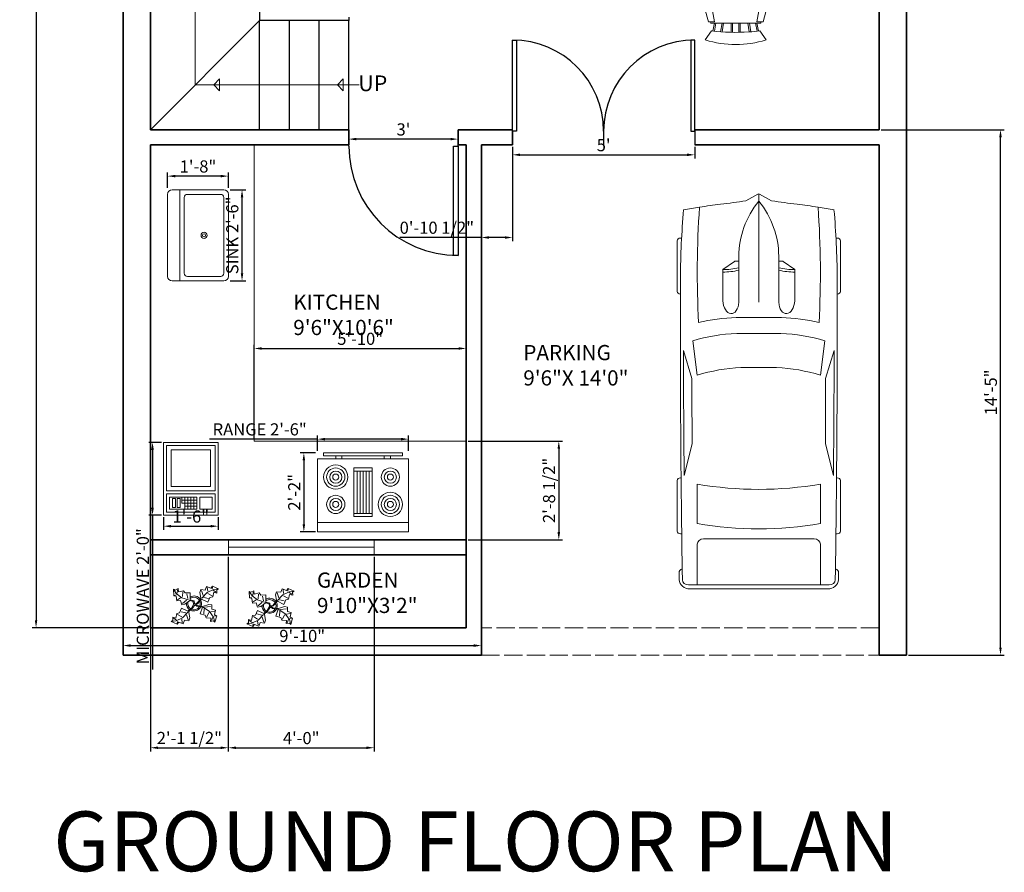
# Model space of a CAD drawing. Units: inches. Extents: x 2170 to 3011, y 1733 to 2338.
# Tile 1 of 5: x 2172 to 2496, y 1733 to 2014. Entities that reach past the tile are written whole.
import ezdxf

# ---------------------------------------------------------------- set-up
doc = ezdxf.new("R2010")
doc.units = ezdxf.units.IN
doc.linetypes.add('ACAD_ISO02W100', pattern=[15, 12, -3])
for name, color, linetype, lineweight in [('A-ANNO-SYMB', 2, 'Continuous', 13), ('A-AREA-IDEN', 4, 'Continuous', 18), ('A-EQPM', 20, 'Continuous', 18), ('A-FLOR-CASE', 20, 'Continuous', 20), ('A-FLOR-FIXT', 20, 'Continuous', 18), ('A-WALL', 7, 'Continuous', 35), ('A-WALL-OVHD', 7, 'ACAD_ISO02W100', 18), ('car', 81, 'Continuous', 13), ('dim', 11, 'Continuous', 18), ('door', 6, 'Continuous', 25), ('furnitures', 20, 'Continuous', 18), ('L-PLNT', 81, 'Continuous', 13), ('stairs', 150, 'Continuous', 25), ('text', 4, 'Continuous', 18), ('window', 3, 'Continuous', 20)]:
    doc.layers.add(name, color=color, linetype=linetype, lineweight=lineweight)
doc.styles.get("Standard").update_dxf_attribs({"font": 'arial.ttf'})
doc.dimstyles.new('ISO-25', dxfattribs={"dimtxt": 4, "dimasz": 2.5, "dimexe": 1.25, "dimexo": 0.625, "dimtad": 1, "dimlunit": 3, "dimtxsty": 'Standard', "dimcen": 2.5, "dimadec": 0, "dimazin": 0, "dimtfac": 1, "dimtmove": 0, "dimatfit": 3, "dimfxl": 1, "dimarcsym": 0})

# ---------------------------------------------------------------- blocks, each defined once
blk = doc.blocks.new('*U4')
for p, q in [((0, 0), (0, -6)), ((40, 0), (40, -6))]:
    blk.add_line(p, q)
blk.add_lwpolyline([(0, 0), (0, 40), (1.75, 40), (1.75, 0)], close=True)
blk.add_arc((0, 0), 40, 0, 90)
blk = doc.blocks.new('*U2')
for p, q in [((0, 0), (0, -6)), ((40, 0), (40, -6))]:
    blk.add_line(p, q)
blk.add_lwpolyline([(0, 0), (0, 40), (1.75, 40), (1.75, 0)], close=True)
blk.add_arc((0, 0), 40, 0, 90)
blk = doc.blocks.new('*U3')
for p, q in [((0, 0), (0, -6)), ((-40, 0), (-40, -6))]:
    blk.add_line(p, q)
blk.add_lwpolyline([(0, 0), (0, 40), (-1.75, 40), (-1.75, 0)], close=True)
blk.add_arc((0, 0), 40, 90, 180)
blk = doc.blocks.new('Range-Oven - 30 in top')
for p, q in [((0, -3), (30, -3)), ((12, -6), (18, -6)), ((13, -20), (13, -6)), ((14, -6), (14, -20)), ((15, -20), (15, -6)), ((16, -6), (16, -20)), ((17, -20), (17, -6)), ((18, -20), (12, -20)), ((6, -24), (6, -25)), ((8, -25), (8, -24)), ((22, -25), (22, -24)), ((24, -24), (24, -25))]:
    blk.add_line(p, q)
for points in [[(0, -24), (0, 0), (30, 0), (30, -24)], [(12, -21), (12, -5), (18, -5), (18, -21)], [(2, -26), (2, -25), (28, -25), (28, -26)]]:
    blk.add_lwpolyline(points, close=True)
for centre, radius in [((6, -9), 4), ((6, -9), 3), ((24, -9), 3), ((6, -9), 2), ((6, -9), 1), ((24, -9), 2), ((24, -9), 1), ((6, -18), 3), ((6, -18), 2), ((24, -18), 4), ((24, -18), 3), ((24, -18), 2), ((6, -18), 1), ((24, -18), 1)]:
    blk.add_circle(centre, radius)
blk = doc.blocks.new('Microwave')
for p, q in [((18, 10), (22, 10)), ((19, 7), (19, 11)), ((20, 11), (20, 7)), ((21, 7), (21, 11)), ((22, 9), (18, 9)), ((18, 8), (22, 8)), ((22, 7), (18, 7)), ((19, 6), (19, 7)), ((20, 7), (20, 6)), ((20, 6), (18, 6))]:
    blk.add_line(p, q)
for points in [[(0, 0), (0, 18), (24, 18), (24, 0)], [(1, 1), (1, 17), (16, 17), (16, 1)], [(17, 1), (17, 17), (23, 17), (23, 1)], [(2.5, 2.5), (2.5, 15.5), (14.5, 15.5), (14.5, 2.5)], [(18, 12), (18, 16), (22, 16), (22, 12)], [(18, 2), (18, 11), (22, 11), (22, 2)], [(18.5, 4.5), (18.5, 5.5), (21.5, 5.5), (21.5, 4.5)], [(18.5, 3), (18.5, 4), (21.5, 4), (21.5, 3)]]:
    blk.add_lwpolyline(points, close=True)
blk = doc.blocks.new('Sink-single - 30 in top')
blk.add_line((-15, -3.999996), (15, -3.999996))
for points in [[(-13.5, 0), (13.5, 0)], [(-15, -18.499996), (-15, -1.5)], [(15, -1.5), (15, -18.499996)], [(-12.5, -5.499996), (12.5, -5.499996)], [(-13.5, -17.499996), (-13.5, -6.499996)], [(13.5, -6.499996), (13.5, -17.499996)], [(12.5, -18.499996), (-12.5, -18.499996)], [(13.5, -19.999996), (-13.5, -19.999996)]]:
    blk.add_lwpolyline(points)
for radius in [1, 0.5]:
    blk.add_circle((0, -11.999996), radius)
for centre, radius, start, end in [((-13.5, -1.5), 1.5, 90, 180), ((13.5, -1.5), 1.5, 0, 90), ((-12.5, -6.499996), 1, 90, 180), ((12.5, -6.499996), 1, 0, 90), ((-13.5, -18.499996), 1.5, 180, 270), ((-12.5, -17.499996), 1, 180, 270), ((12.5, -17.499996), 1, 270, 0), ((13.5, -18.499996), 1.5, 270, 0)]:
    blk.add_arc(centre, radius, start, end)
blk = doc.blocks.new('Plant - Rubber or Philodendron')
for p, q in [((-16.2005, 11.4774), (-13.9899, 8.1064)), ((-16.2005, 11.4774), (-14.8639, 10.7964)), ((-16.0159, 6.3329), (-16.2005, 11.4774)), ((-14.8639, 10.7964), (-12.6195, 11.8975)), ((-13.9899, 8.1064), (-9.5434, 4.7185)), ((-13.3174, 8.325), (-13.0735, 11.0065)), ((-12.6195, 11.8975), (-12.1909, 9.4345)), ((-12.1909, 9.4345), (-8.3829, 10.3)), ((-8.8369, 9.409), (-9.0894, 5.6095)), ((-8.3829, 10.3), (-7.0549, 8.501)), ((-7.0549, 8.501), (-3.0284, 8.6941)), ((-4.8529, 4.012), (-5.7184, 7.82)), ((-3.0284, 8.6941), (-3.0709, 3.1041)), ((4.6914, 8.8812), (5.3859, 11.2828)), ((4.6914, 8.8812), (5.5014, 4.4831)), ((5.3859, 11.2828), (8.8871, 10.7908)), ((5.9878, 10.4842), (7.1971, 6.3869)), ((10.3916, 8.7942), (6.2847, 4.4028)), ((8.8871, 10.7908), (9.9809, 13.4933)), ((9.9809, 13.4933), (13.3837, 12.301)), ((15.3859, 11.3055), (10.3916, 8.7942)), ((10.5828, 12.6946), (10.8893, 9.7953)), ((14.2977, 6.1031), (10.9934, 7.9956)), ((13.3837, 12.301), (14.68, 13.9039)), ((14.5816, 13.2037), (14.3848, 11.8033)), ((14.68, 13.9039), (19.3848, 11.8146)), ((15.7909, 9.1065), (14.8995, 5.3044)), ((15.2875, 10.6053), (17.5907, 9.2105)), ((19.3848, 11.8146), (15.3859, 11.3055)), ((18.1925, 8.4119), (15.7909, 9.1065)), ((19.3848, 11.8146), (18.1868, 10.9119)), ((18.1868, 10.9119), (18.1925, 8.4119)), ((-14.0069, 5.8704), (-16.0159, 6.3329)), ((-15.3434, 6.5514), (-13.9984, 6.9884)), ((-13.5868, 2.2894), (-14.0069, 5.8704)), ((-10.6784, 2.491), (-13.5868, 2.2894)), ((-13.1329, 3.1804), (-10.6614, 4.727)), ((-9.5858, -0.8715), (-10.6784, 2.491)), ((-9.5434, 4.7185), (-4.1917, 2.9888)), ((-9.1318, 0.0195), (-5.9793, 2.9025)), ((-7.1228, -0.443), (-3.5248, 2.2131)), ((-3.5248, 2.2131), (-3.3011, 2.4355)), ((-3.3011, 2.4355), (-0.5306, 1.7947)), ((-3.0709, 3.1041), (0.0797, 2.3163)), ((-0.5306, 1.7947), (-0.2255, -0.5527)), ((-0.5306, 1.7947), (-0.5306, 1.7947)), ((0.0797, 2.3163), (0.4866, -0.031)), ((0.4866, -0.031), (2.1141, 0.2298)), ((2.1141, 0.2298), (5.4346, 3.9146)), ((6.1032, 3.6844), (2.8262, -0.031)), ((5.4346, 3.9146), (5.5014, 4.4831)), ((11.1089, 1.1958), (6.1032, 3.6844)), ((7.7005, 4.8881), (11.5025, 3.9967)), ((12.7005, 4.8994), (11.1089, 1.1958)), ((14.8995, 5.3044), (12.7005, 4.8994)), ((-14.4141, -11.4699), (-13.5228, -7.6679)), ((-13.5228, -7.6679), (-11.3237, -7.2629)), ((-11.3237, -7.2629), (-9.7321, -3.5593)), ((-6.3237, -7.2516), (-10.1257, -6.3602)), ((-9.7321, -3.5593), (-4.7264, -6.0479)), ((-7.1228, -0.443), (-9.5858, -0.8715)), ((-9.0148, -11.1577), (-4.9047, -6.8122)), ((-2.019, -3.6148), (-4.7264, -6.0479)), ((-4.1246, -6.8466), (-4.0579, -6.2781)), ((-3.3146, -11.2447), (-4.1246, -6.8466)), ((-4.0579, -6.2781), (-0.9375, -3.1608)), ((-2.019, -3.6148), (-0.2255, -0.5527)), ((-0.9375, -3.1608), (0.5883, -0.8135)), ((0.5883, -0.8135), (2.2447, -2.0916)), ((2.8262, -0.031), (1.3003, -0.5527)), ((1.3003, -0.5527), (2.4193, -1.4655)), ((2.2447, -2.0916), (6.7108, -2.6626)), ((2.4193, -1.4655), (6.895, -2.1175)), ((4.943, -7.9659), (6.7108, -2.6626)), ((11.6605, -0.5413), (6.895, -2.1175)), ((12.3677, -6.1981), (7.219, -2.6772)), ((8.125, -4.0768), (7.7715, -7.9659)), ((8.3544, -2.7453), (13.1973, -2.1704)), ((10.2463, -10.4408), (11.6605, -6.9053)), ((11.6605, -0.5413), (14.1354, -0.8948)), ((15.5496, -10.7943), (12.3677, -6.1981)), ((16.2567, -5.8446), (13.4283, -6.5517)), ((14.1354, -0.8948), (14.1354, -4.4304)), ((14.1354, -4.4304), (16.9638, -5.1375)), ((16.9638, -5.1375), (16.2567, -8.673)), ((-18.008, -14.1781), (-16.8101, -13.2754)), ((-18.008, -14.1781), (-14.0091, -13.669)), ((-13.3032, -16.2674), (-18.008, -14.1781)), ((-16.8157, -10.7754), (-14.4141, -11.4699)), ((-16.8101, -13.2754), (-16.8157, -10.7754)), ((-13.9107, -12.9688), (-16.2139, -11.574)), ((-14.0091, -13.669), (-9.0148, -11.1577)), ((-12.0069, -14.6645), (-13.3032, -16.2674)), ((-13.2048, -15.5672), (-13.008, -14.1668)), ((-12.921, -8.4665), (-9.6166, -10.359)), ((-8.6042, -15.8568), (-12.0069, -14.6645)), ((-9.206, -15.0581), (-9.5126, -12.1588)), ((-7.5103, -13.1543), (-8.6042, -15.8568)), ((-4.0092, -13.6463), (-7.5103, -13.1543)), ((-4.611, -12.8477), (-5.8203, -8.7504)), ((-3.3146, -11.2447), (-4.0092, -13.6463)), ((8.8321, -9.0266), (4.943, -7.9659)), ((9.5392, -11.1479), (8.8321, -9.0266)), ((13.4283, -11.5015), (9.5392, -11.1479)), ((13.0748, -13.9763), (13.4283, -11.5015)), ((15.5496, -13.6228), (13.0748, -13.9763)), ((14.8425, -10.7943), (13.7819, -13.2692)), ((16.6103, -14.6834), (15.5496, -10.7943)), ((16.6103, -14.6834), (15.5496, -13.6228)), ((17.3174, -9.7337), (15.9032, -9.7337)), ((16.2567, -8.673), (18.0245, -9.7337)), ((18.0245, -9.7337), (16.6103, -14.6834))]:
    blk.add_line(p, q)
for centre, radius, start, end in [((0.0308, 0.1664), 6, 178.6147, 235.1169), ((0.0308, 0.1664), 5, 168.1647, 238.6725), ((0, 0), 6.1275, 34.37569, 120.1028), ((-0.0601, -0.2075), 5.2461, 33.82192, 124.9414), ((-0.2664, 0.1682), 5.2775, 338.4094, 20.03007), ((-0.098, 0.1364), 6.1288, 341.2017, 26.09184), ((-0.0234, 0.3825), 6.1492, 242.5812, 331.2714), ((-0.1102, 0.4886), 5.2883, 247.3711, 327.472)]:
    blk.add_arc(centre, radius, start, end)
blk = doc.blocks.new('Chair - Rocking')
for p, q in [((-8, -4.5), (-10, -1.5)), ((8, -4.5), (10, -1.5)), ((-7.5, -4.5), (-7, -7)), ((-6.5, -7), (-7.02225, -4.43)), ((-4.5, -7), (-4.96674, -4.19951)), ((-4, -7), (-4.40532, -4.16272)), ((-1.5, -4.05012), (-1.5, -7)), ((-1, -7), (-1, -4.05012)), ((1, -7), (1, -4.04655)), ((1.5, -4.05012), (1.5, -7)), ((4, -7), (4.40187, -4.18694)), ((4.5, -7), (4.96761, -4.19437)), ((6.5, -7), (7, -4.4057)), ((7.5, -4.5), (7, -7)), ((-9, -7.5), (-12, -18.49999)), ((-7, -7.5), (-9, -7.5)), ((-9, -18.49999), (-7, -7.5)), ((-8.23428, -6.99939), (-8.3093, -7.47958)), ((-8.23041, -7), (8.23915, -7)), ((7, -7.5), (9, -7.5)), ((9, -18.49999), (7, -7.5)), ((8.31071, -7.48854), (8.23449, -7.00073)), ((9, -7.5), (12, -18.49999)), ((-10.36644, -20.64523), (-10.5, -21.49999)), ((-9, -22.49999), (-9.5, -26.49999)), ((0, -22.49999), (-9.5, -22.49999)), ((-8, -26.49999), (-7.5, -22.49999)), ((0, -22.49999), (9.5, -22.49999)), ((8, -26.49999), (7.5, -22.49999)), ((9, -22.49999), (9.5, -26.49999)), ((10.5, -21.49999), (10.3575, -20.58798)), ((-9.5, -26.49999), (-8, -26.49999)), ((9.5, -26.49999), (8, -26.49999))]:
    blk.add_line(p, q)
for centre, radius, start, end in [((0, -34.08333), 34.08333, 72.93847, 107.0615), ((0, -68.25004), 64.25, 93.92211, 97.15267), ((0, -68.25004), 64.25, 82.84733, 93.92211), ((-10.5, -18.99999), 1.58114, 161.5651, 18.43495), ((10.5, -18.99999), 1.58114, 161.5651, 18.43495), ((-9.5, -21.49999), 1, 180, 270), ((9.5, -21.49999), 1, 270, 0)]:
    blk.add_arc(centre, radius, start, end)
blk = doc.blocks.new('*U21')
for p, q in [((46.55, 38.89), (22.35, 38.89)), ((136.7, 38.89), (160.9, 38.89)), ((21.1, 37.41), (21.1, 36.83)), ((47.8, 37.39), (47.8, 37.41)), ((87.99, 31.87), (74.76, 35.92)), ((134.31, 35.6), (119.29, 31.78)), ((135.45, 37.07), (135.45, 37.41)), ((162.15, 37.41), (162.15, 36.77)), ((186.47, -33.5), (186.47, 33.5)), ((70.03, 31.54), (86.41, 29.35)), ((138.42, 29.35), (157.25, 29.35)), ((186.47, 29.35), (167.01, 29.35)), ((188.4, -32.76), (188.4, 32.76)), ((164.52, 26.39), (164.52, -26.39)), ((32.27, 11.63), (36.13, 17.17)), ((36.13, 17.17), (50.94, 17.17)), ((29.77, 9.51), (51.68, 9.51)), ((32.12, 9.51), (32.12, 11.15)), ((58.92, -10.77), (58.92, 10.77)), ((66.55, -10.53), (66.55, 10.53)), ((186.47, -10.53), (186.47, 10.53)), ((3.27, 6.13), (0.1, 0.41)), ((82.74, 8.5), (82.74, -8.5)), ((0, 0), (51.68, 0)), ((0.1, -0.41), (3.27, -6.13)), ((29.77, -9.51), (51.68, -9.51)), ((32.12, -9.51), (32.12, -11.15)), ((32.27, -11.63), (36.13, -17.17)), ((36.13, -17.17), (50.94, -17.17)), ((86.41, -29.35), (70.03, -31.54)), ((87.99, -31.87), (74.76, -35.92)), ((134.31, -35.6), (119.29, -31.78)), ((157.25, -29.35), (138.42, -29.35)), ((167.01, -29.35), (186.47, -29.35)), ((21.1, -37.41), (21.1, -36.83)), ((47.8, -37.39), (47.8, -37.41)), ((135.45, -37.07), (135.45, -37.41)), ((162.15, -37.41), (162.15, -36.77)), ((46.55, -38.89), (22.35, -38.89)), ((136.7, -38.89), (160.9, -38.89))]:
    blk.add_line(p, q)
for centre, major_axis, ratio, start_param, end_param in [((22.35, 37.41), (0, -1.48), 0.842304, 3.141593, 4.712389), ((46.55, 37.41), (0, 1.48), 0.842304, -1.570796, 0), ((136.7, 37.41), (0, -1.48), 0.842304, 3.141593, 4.712389), ((160.9, 37.41), (0, 1.48), 0.842304, -1.570796, 0), ((180.63, 35.84), (0, 2.22), 0.842304, -0.013017, 1.249894), ((64.48, -10556.36), (0, 10595.31), 0.842304, -0.013397, -0.013017), ((183.98, 32.76), (0, -5.25), 0.842304, 1.570796, 3.128196), ((266.03, -27.52), (0, 313.31), 0.842304, 1.367076, 1.39176), ((41.19, -490.86), (0, 528.23), 0.842304, 0.00281, 0.075598), ((64.48, -10555.62), (0, 10593.03), 0.842304, -0.013397, 0.002797), ((64.48, -10555.62), (0, -10591.55), 0.842304, 3.133765, 3.140441), ((183.98, 33.5), (0, -2.96), 0.842304, 1.570796, 3.128196), ((259.18, -27.52), (0, -305.3), 0.842304, 4.528606, 4.561838), ((37.47, -593.96), (0, -623.33), 0.842304, 3.096046, 3.200911), ((134.4, 5.39), (0, -89.78), 0.842304, 4.449482, 4.652344), ((135.29, 5.39), (0, 81.77), 0.842304, 1.245306, 1.50788), ((149.6, 2.8), (0, -79.58), 0.842304, 4.372215, 4.640744), ((95.79, -3666.35), (0, -3698.24), 0.842304, 3.134049, 3.144098), ((17.08, 0), (0, 147.02), 0.842304, 4.511394, 4.913384), ((35.91, 0), (0, 147.02), 0.842304, 4.511394, 4.913384), ((167.01, 26.39), (0, 2.96), 0.842304, 0, 1.570796), ((-204.49, 52.4), (0, -250.96), 0.842304, 1.385369, 1.434372), ((13.04, 17.01), (0, 27.42), 0.842304, 4.435146, 4.718221), ((14.2, 17.01), (0, 27.42), 0.842304, 4.435146, 4.718221), ((50.79, 13.34), (6.34, -0.36), 0.603834, -1.395552, 1.581315), ((29.77, -46.66), (0, 56.17), 0.842304, 0, 0.590319), ((32.75, 11.15), (0, 0.74), 0.842304, 0.879714, 1.570796), ((0.62, 0), (0, -0.74), 0.842304, 4.131459, 5.293319), ((29.77, 46.66), (0, 56.17), 0.842304, 2.551274, 3.141593), ((-204.49, -52.4), (0, 250.96), 0.842304, -1.434372, -1.385369), ((149.6, -2.8), (0, -79.58), 0.842304, -1.499151, -1.230623), ((32.75, -11.15), (0, -0.74), 0.842304, 4.712389, 5.403472), ((13.04, -17.01), (0, -27.42), 0.842304, 1.564964, 1.848039), ((14.2, -17.01), (0, -27.42), 0.842304, 1.564964, 1.848039), ((134.4, -5.39), (0, -89.78), 0.842304, -1.510751, -1.307889), ((135.29, -5.39), (0, -81.77), 0.842304, -1.50788, -1.245306), ((259.18, 27.52), (0, 305.3), 0.842304, 1.721348, 1.754579), ((167.01, -26.39), (0, -2.96), 0.842304, 4.712389, 6.283185), ((266.03, 27.52), (0, 313.31), 0.842304, 1.749832, 1.774517), ((37.47, 593.96), (0, -623.33), 0.842304, -0.059319, 0.045547), ((95.79, 3666.35), (0, -3698.24), 0.842304, -0.002505, 0.007544), ((183.98, -32.76), (0, -5.25), 0.842304, 0.013397, 1.570796), ((41.19, 490.86), (0, -528.23), 0.842304, -0.075598, -0.00281), ((22.35, -37.41), (0, 1.48), 0.842304, 1.570796, 3.141593), ((64.48, 10555.62), (0, 10593.03), 0.842304, 3.138796, 3.15499), ((46.55, -37.41), (0, -1.48), 0.842304, 0, 1.570796), ((64.48, 10555.62), (0, -10591.55), 0.842304, 0.001152, 0.007828), ((136.7, -37.41), (0, -1.48), 0.842304, -1.570796, 0), ((160.9, -37.41), (0, 1.48), 0.842304, 3.141593, 4.712389), ((180.63, -35.84), (0, -2.22), 0.842304, -1.249894, 0.013017), ((183.98, -33.5), (0, 2.96), 0.842304, 3.15499, 4.712389), ((64.48, 10556.36), (0, 10595.31), 0.842304, 3.15461, 3.15499)]:
    blk.add_ellipse(centre, major_axis=major_axis, ratio=ratio, start_param=start_param, end_param=end_param)
at = {"extrusion": (0, 0, -1)}
blk.add_ellipse((50.79, -13.34), major_axis=(6.34, 0.36), ratio=0.603834, start_param=-1.395552, end_param=1.581315, dxfattribs=at)
blk = doc.blocks.new('*D23')
at = {"layer": 'Defpoints', "color": 0, "transparency": 16777216}
for p in [(2215.17, 2293.31), (2177.52, 1813.31), (2215.17, 1813.31)]:
    blk.add_point(p, dxfattribs=at)
at = {"layer": 'dim', "color": 0, "lineweight": -2, "transparency": 16777216}
for p, q in [((2214.54, 2293.31), (2176.27, 2293.31)), ((2177.52, 2290.81), (2177.52, 1815.81)), ((2214.54, 1813.31), (2176.27, 1813.31))]:
    blk.add_line(p, q, dxfattribs=at)
at = {"layer": 'dim', "color": 0, "transparency": 16777216}
for points in [[(2177.11, 2290.81), (2177.94, 2290.81), (2177.52, 2293.31)], [(2177.11, 1815.81), (2177.94, 1815.81), (2177.52, 1813.31)]]:
    blk.add_solid(points, dxfattribs=at)
at = {"layer": 'dim', "color": 0, "transparency": 16777216, "insert": (2174.86, 2053.31), "char_height": 4, "attachment_point": 5, "rotation": 90}
blk.add_mtext("40'", dxfattribs=at)
blk = doc.blocks.new('*D27')
at = {"layer": 'Defpoints', "color": 0, "transparency": 16777216}
for p in [(2280.51, 1974.2), (2280.51, 1972.31), (2316.51, 1972.31)]:
    blk.add_point(p, dxfattribs=at)
at = {"layer": 'dim', "color": 0, "lineweight": -2, "transparency": 16777216}
for p, q in [((2280.51, 1972.93), (2280.51, 1975.45)), ((2316.51, 1972.93), (2316.51, 1975.45)), ((2314.01, 1974.2), (2283.01, 1974.2))]:
    blk.add_line(p, q, dxfattribs=at)
at = {"layer": 'dim', "color": 0, "transparency": 16777216}
for points in [[(2283.01, 1974.62), (2283.01, 1973.79), (2280.51, 1974.2)], [(2314.01, 1974.62), (2314.01, 1973.79), (2316.51, 1974.2)]]:
    blk.add_solid(points, dxfattribs=at)
at = {"layer": 'dim', "color": 0, "transparency": 16777216, "insert": (2298.51, 1976.87), "char_height": 4, "attachment_point": 5}
blk.add_mtext("3'", dxfattribs=at)
blk = doc.blocks.new('*D28')
at = {"layer": 'Defpoints', "color": 0, "transparency": 16777216}
for p in [(2334.43, 1972.31), (2394.43, 1972.31), (2394.43, 1969.03)]:
    blk.add_point(p, dxfattribs=at)
at = {"layer": 'dim', "color": 0, "lineweight": -2, "transparency": 16777216}
for p, q in [((2334.43, 1971.68), (2334.43, 1967.78)), ((2394.43, 1971.68), (2394.43, 1967.78)), ((2336.93, 1969.03), (2391.93, 1969.03))]:
    blk.add_line(p, q, dxfattribs=at)
at = {"layer": 'dim', "color": 0, "transparency": 16777216}
for points in [[(2336.93, 1969.45), (2336.93, 1968.62), (2334.43, 1969.03)], [(2391.93, 1969.45), (2391.93, 1968.62), (2394.43, 1969.03)]]:
    blk.add_solid(points, dxfattribs=at)
at = {"layer": 'dim', "color": 0, "transparency": 16777216, "insert": (2364.43, 1971.69), "char_height": 4, "attachment_point": 5}
blk.add_mtext("5'", dxfattribs=at)
blk = doc.blocks.new('*D29')
at = {"layer": 'Defpoints', "color": 0, "transparency": 16777216}
for p in [(2206.17, 1813.31), (2324.17, 1813.31), (2324.17, 1807.45)]:
    blk.add_point(p, dxfattribs=at)
at = {"layer": 'dim', "color": 0, "lineweight": -2, "transparency": 16777216}
for p, q in [((2206.17, 1812.68), (2206.17, 1806.2)), ((2324.17, 1812.68), (2324.17, 1806.2)), ((2208.67, 1807.45), (2321.67, 1807.45))]:
    blk.add_line(p, q, dxfattribs=at)
at = {"layer": 'dim', "color": 0, "transparency": 16777216}
for points in [[(2208.67, 1807.87), (2208.67, 1807.03), (2206.17, 1807.45)], [(2321.67, 1807.87), (2321.67, 1807.03), (2324.17, 1807.45)]]:
    blk.add_solid(points, dxfattribs=at)
at = {"layer": 'dim', "color": 0, "transparency": 16777216, "insert": (2265.17, 1810.12), "char_height": 4, "attachment_point": 5}
blk.add_mtext('9\'-10"', dxfattribs=at)
blk = doc.blocks.new('STAIR-UP-PATH')
for p, q in [((16.56, 133.24), (16.56, 137.12)), ((16.56, 137.12), (18.45, 135.18)), ((76.31, 133.24), (76.31, 137.12)), ((76.31, 137.12), (78.21, 135.18)), ((1.94, 1.94), (1.94, 135.18)), ((1.94, 135.18), (83.94, 135.18)), ((16.56, 133.24), (18.45, 135.18)), ((76.31, 133.24), (78.21, 135.18)), ((0, 122.86), (1.94, 124.75)), ((3.88, 122.86), (1.94, 124.75)), ((3.88, 122.86), (0, 122.86)), ((0, 41.63), (1.94, 43.52)), ((3.88, 41.63), (1.94, 43.52)), ((3.88, 41.63), (0, 41.63)), ((9.93, 3.88), (8.04, 1.94)), ((9.93, 3.88), (9.93, 0)), ((50.68, 3.88), (48.79, 1.94)), ((50.68, 3.88), (50.68, 0)), ((55.9, 1.94), (1.94, 1.94)), ((9.93, 0), (8.04, 1.94)), ((50.68, 0), (48.79, 1.94))]:
    blk.add_line(p, q)
blk = doc.blocks.new('*D68')
at = {"layer": 'Defpoints', "color": 0, "transparency": 16777216}
for p in [(2270.21, 1875.42), (2270.21, 1870.92), (2300.21, 1870.92)]:
    blk.add_point(p, dxfattribs=at)
at = {"layer": 'dim', "color": 0, "lineweight": -2, "transparency": 16777216}
for p, q in [((2270.21, 1875.42), (2234.61, 1875.42)), ((2270.21, 1871.55), (2270.21, 1876.67)), ((2297.71, 1875.42), (2272.71, 1875.42)), ((2300.21, 1871.55), (2300.21, 1876.67))]:
    blk.add_line(p, q, dxfattribs=at)
at = {"layer": 'dim', "color": 0, "transparency": 16777216}
for points in [[(2272.71, 1875.84), (2272.71, 1875), (2270.21, 1875.42)], [(2297.71, 1875.84), (2297.71, 1875), (2300.21, 1875.42)]]:
    blk.add_solid(points, dxfattribs=at)
at = {"layer": 'dim', "color": 0, "transparency": 16777216, "insert": (2251.16, 1878.11), "char_height": 4, "attachment_point": 5}
blk.add_mtext('RANGE 2\'-6"', dxfattribs=at)
blk = doc.blocks.new('*D69')
at = {"layer": 'Defpoints', "color": 0, "transparency": 16777216}
for p in [(2270.21, 1870.92), (2265.71, 1844.92), (2270.21, 1844.92)]:
    blk.add_point(p, dxfattribs=at)
at = {"layer": 'dim', "color": 0, "lineweight": -2, "transparency": 16777216}
for p, q in [((2269.59, 1870.92), (2264.46, 1870.92)), ((2265.71, 1868.42), (2265.71, 1847.42)), ((2269.59, 1844.92), (2264.46, 1844.92))]:
    blk.add_line(p, q, dxfattribs=at)
at = {"layer": 'dim', "color": 0, "transparency": 16777216}
for points in [[(2265.3, 1868.42), (2266.13, 1868.42), (2265.71, 1870.92)], [(2265.3, 1847.42), (2266.13, 1847.42), (2265.71, 1844.92)]]:
    blk.add_solid(points, dxfattribs=at)
at = {"layer": 'dim', "color": 0, "transparency": 16777216, "insert": (2263.08, 1857.92), "char_height": 4, "attachment_point": 5, "rotation": 90}
blk.add_mtext('2\'-2"', dxfattribs=at)
blk = doc.blocks.new('*D70')
at = {"layer": 'Defpoints', "color": 0, "transparency": 16777216}
for p in [(2219.48, 1874.36), (2215.88, 1850.36), (2219.48, 1850.36)]:
    blk.add_point(p, dxfattribs=at)
at = {"layer": 'dim', "color": 0, "lineweight": -2, "transparency": 16777216}
for p, q in [((2218.86, 1874.36), (2214.63, 1874.36)), ((2215.88, 1871.86), (2215.88, 1852.86)), ((2218.86, 1850.36), (2214.63, 1850.36)), ((2215.88, 1850.36), (2215.88, 1799.53))]:
    blk.add_line(p, q, dxfattribs=at)
at = {"layer": 'dim', "color": 0, "transparency": 16777216}
for points in [[(2215.46, 1871.86), (2216.3, 1871.86), (2215.88, 1874.36)], [(2215.46, 1852.86), (2216.3, 1852.86), (2215.88, 1850.36)]]:
    blk.add_solid(points, dxfattribs=at)
at = {"layer": 'dim', "color": 0, "transparency": 16777216, "insert": (2213.19, 1823.69), "char_height": 4, "attachment_point": 5, "rotation": 90}
blk.add_mtext('MICROWAVE 2\'-0"', dxfattribs=at)
blk = doc.blocks.new('*D71')
at = {"layer": 'Defpoints', "color": 0, "transparency": 16777216}
for p in [(2219.48, 1850.36), (2237.48, 1850.36), (2237.48, 1846.76)]:
    blk.add_point(p, dxfattribs=at)
at = {"layer": 'dim', "color": 0, "lineweight": -2, "transparency": 16777216}
for p, q in [((2219.48, 1849.73), (2219.48, 1845.51)), ((2237.48, 1849.73), (2237.48, 1845.51)), ((2221.98, 1846.76), (2234.98, 1846.76))]:
    blk.add_line(p, q, dxfattribs=at)
at = {"layer": 'dim', "color": 0, "transparency": 16777216}
for points in [[(2221.98, 1847.18), (2221.98, 1846.34), (2219.48, 1846.76)], [(2234.98, 1847.18), (2234.98, 1846.34), (2237.48, 1846.76)]]:
    blk.add_solid(points, dxfattribs=at)
at = {"layer": 'dim', "color": 0, "transparency": 16777216, "insert": (2228.48, 1849.43), "char_height": 4, "attachment_point": 5}
blk.add_mtext('1\'-6"', dxfattribs=at)
blk = doc.blocks.new('*D72')
at = {"layer": 'Defpoints', "color": 0, "transparency": 16777216}
for p in [(2240.85, 1957.51), (2245.35, 1957.51), (2240.85, 1927.51)]:
    blk.add_point(p, dxfattribs=at)
at = {"layer": 'dim', "color": 0, "lineweight": -2, "transparency": 16777216}
for p, q in [((2241.48, 1957.51), (2246.6, 1957.51)), ((2245.35, 1930.01), (2245.35, 1955.01)), ((2241.48, 1927.51), (2246.6, 1927.51))]:
    blk.add_line(p, q, dxfattribs=at)
at = {"layer": 'dim', "color": 0, "transparency": 16777216}
for points in [[(2244.93, 1955.01), (2245.77, 1955.01), (2245.35, 1957.51)], [(2244.93, 1930.01), (2245.77, 1930.01), (2245.35, 1927.51)]]:
    blk.add_solid(points, dxfattribs=at)
at = {"layer": 'dim', "color": 0, "transparency": 16777216, "insert": (2242.66, 1942.51), "char_height": 4, "attachment_point": 5, "rotation": 90}
blk.add_mtext('SINK 2\'-6"', dxfattribs=at)
blk = doc.blocks.new('*D73')
at = {"layer": 'Defpoints', "color": 0, "transparency": 16777216}
for p in [(2220.85, 1962.01), (2220.85, 1957.51), (2240.85, 1957.51)]:
    blk.add_point(p, dxfattribs=at)
at = {"layer": 'dim', "color": 0, "lineweight": -2, "transparency": 16777216}
for p, q in [((2220.85, 1958.14), (2220.85, 1963.26)), ((2238.35, 1962.01), (2223.35, 1962.01)), ((2240.85, 1958.14), (2240.85, 1963.26))]:
    blk.add_line(p, q, dxfattribs=at)
at = {"layer": 'dim', "color": 0, "transparency": 16777216}
for points in [[(2223.35, 1962.43), (2223.35, 1961.6), (2220.85, 1962.01)], [(2238.35, 1962.43), (2238.35, 1961.6), (2240.85, 1962.01)]]:
    blk.add_solid(points, dxfattribs=at)
at = {"layer": 'dim', "color": 0, "transparency": 16777216, "insert": (2230.85, 1964.68), "char_height": 4, "attachment_point": 5}
blk.add_mtext('1\'-8"', dxfattribs=at)
blk = doc.blocks.new('*D90')
at = {"layer": 'Defpoints', "color": 0, "transparency": 16777216}
for p in [(2240.84, 1837.31), (2288.84, 1837.31), (2288.84, 1773.81)]:
    blk.add_point(p, dxfattribs=at)
at = {"layer": 'dim', "color": 0, "lineweight": -2, "transparency": 16777216}
for p, q in [((2240.84, 1836.68), (2240.84, 1772.56)), ((2288.84, 1836.68), (2288.84, 1772.56)), ((2243.34, 1773.81), (2286.34, 1773.81))]:
    blk.add_line(p, q, dxfattribs=at)
at = {"layer": 'dim', "color": 0, "transparency": 16777216}
for points in [[(2243.34, 1774.22), (2243.34, 1773.39), (2240.84, 1773.81)], [(2286.34, 1774.22), (2286.34, 1773.39), (2288.84, 1773.81)]]:
    blk.add_solid(points, dxfattribs=at)
at = {"layer": 'dim', "color": 0, "transparency": 16777216, "insert": (2264.84, 1776.47), "char_height": 4, "attachment_point": 5}
blk.add_mtext('4\'-0"', dxfattribs=at)
blk = doc.blocks.new('*D91')
at = {"layer": 'Defpoints', "color": 0, "transparency": 16777216}
for p in [(2215.17, 1837.31), (2240.84, 1837.31), (2240.84, 1773.81)]:
    blk.add_point(p, dxfattribs=at)
at = {"layer": 'dim', "color": 0, "lineweight": -2, "transparency": 16777216}
for p, q in [((2215.17, 1836.68), (2215.17, 1772.56)), ((2240.84, 1836.68), (2240.84, 1772.56)), ((2217.67, 1773.81), (2238.34, 1773.81))]:
    blk.add_line(p, q, dxfattribs=at)
at = {"layer": 'dim', "color": 0, "transparency": 16777216}
for points in [[(2217.67, 1774.22), (2217.67, 1773.39), (2215.17, 1773.81)], [(2238.34, 1774.22), (2238.34, 1773.39), (2240.84, 1773.81)]]:
    blk.add_solid(points, dxfattribs=at)
at = {"layer": 'dim', "color": 0, "transparency": 16777216, "insert": (2228.01, 1776.5), "char_height": 4, "attachment_point": 5}
blk.add_mtext('2\'-1 1/2"', dxfattribs=at)
blk = doc.blocks.new('*D102')
at = {"layer": 'Defpoints', "color": 0, "transparency": 16777216}
for p in [(2455.17, 1977.31), (2495.13, 1977.31), (2464.17, 1804.31)]:
    blk.add_point(p, dxfattribs=at)
at = {"layer": 'dim', "color": 0, "lineweight": -2, "transparency": 16777216}
for p, q in [((2455.79, 1977.31), (2496.38, 1977.31)), ((2495.13, 1806.81), (2495.13, 1974.81)), ((2464.79, 1804.31), (2496.38, 1804.31))]:
    blk.add_line(p, q, dxfattribs=at)
at = {"layer": 'dim', "color": 0, "transparency": 16777216}
for points in [[(2494.72, 1974.81), (2495.55, 1974.81), (2495.13, 1977.31)], [(2494.72, 1806.81), (2495.55, 1806.81), (2495.13, 1804.31)]]:
    blk.add_solid(points, dxfattribs=at)
at = {"layer": 'dim', "color": 0, "transparency": 16777216, "insert": (2492.47, 1890.81), "char_height": 4, "attachment_point": 5, "rotation": 90}
blk.add_mtext('14\'-5"', dxfattribs=at)
blk = doc.blocks.new('*D105')
at = {"layer": 'Defpoints', "color": 0, "transparency": 16777216}
for p in [(2324.17, 1972.31), (2334.43, 1972.31), (2324.17, 1941.81)]:
    blk.add_point(p, dxfattribs=at)
at = {"layer": 'dim', "color": 0, "lineweight": -2, "transparency": 16777216}
for p, q in [((2324.17, 1971.68), (2324.17, 1940.56)), ((2334.43, 1971.68), (2334.43, 1940.56)), ((2324.17, 1941.81), (2297.36, 1941.81)), ((2331.93, 1941.81), (2326.67, 1941.81))]:
    blk.add_line(p, q, dxfattribs=at)
at = {"layer": 'dim', "color": 0, "transparency": 16777216}
for points in [[(2326.67, 1942.22), (2326.67, 1941.39), (2324.17, 1941.81)], [(2331.93, 1942.22), (2331.93, 1941.39), (2334.43, 1941.81)]]:
    blk.add_solid(points, dxfattribs=at)
at = {"layer": 'dim', "color": 0, "transparency": 16777216, "insert": (2309.51, 1944.5), "char_height": 4, "attachment_point": 5}
blk.add_mtext('0\'-10 1/2"', dxfattribs=at)
blk = doc.blocks.new('*D107')
at = {"layer": 'Defpoints', "color": 0, "transparency": 16777216}
for p in [(2319.17, 1905.27), (2249.34, 1874.77), (2319.17, 1874.77)]:
    blk.add_point(p, dxfattribs=at)
at = {"layer": 'dim', "color": 0, "lineweight": -2, "transparency": 16777216}
for p, q in [((2249.34, 1875.4), (2249.34, 1906.52)), ((2251.84, 1905.27), (2316.67, 1905.27)), ((2319.17, 1875.4), (2319.17, 1906.52))]:
    blk.add_line(p, q, dxfattribs=at)
at = {"layer": 'dim', "color": 0, "transparency": 16777216}
for points in [[(2251.84, 1905.69), (2251.84, 1904.86), (2249.34, 1905.27)], [(2316.67, 1905.69), (2316.67, 1904.86), (2319.17, 1905.27)]]:
    blk.add_solid(points, dxfattribs=at)
at = {"layer": 'dim', "color": 0, "transparency": 16777216, "insert": (2284.26, 1907.94), "char_height": 4, "attachment_point": 5}
blk.add_mtext('5\'-10"', dxfattribs=at)
blk = doc.blocks.new('*D108')
at = {"layer": 'Defpoints', "color": 0, "transparency": 16777216}
for p in [(2319.17, 1874.77), (2319.17, 1842.31), (2349.67, 1842.31)]:
    blk.add_point(p, dxfattribs=at)
at = {"layer": 'dim', "color": 0, "lineweight": -2, "transparency": 16777216}
for p, q in [((2319.79, 1874.77), (2350.92, 1874.77)), ((2349.67, 1872.27), (2349.67, 1844.81)), ((2319.79, 1842.31), (2350.92, 1842.31))]:
    blk.add_line(p, q, dxfattribs=at)
at = {"layer": 'dim', "color": 0, "transparency": 16777216}
for points in [[(2349.25, 1872.27), (2350.09, 1872.27), (2349.67, 1874.77)], [(2349.25, 1844.81), (2350.09, 1844.81), (2349.67, 1842.31)]]:
    blk.add_solid(points, dxfattribs=at)
at = {"layer": 'dim', "color": 0, "transparency": 16777216, "insert": (2346.98, 1858.54), "char_height": 4, "attachment_point": 5, "rotation": 90}
blk.add_mtext('2\'-8 1/2"', dxfattribs=at)

msp = doc.modelspace()

# ---------------------------------------------------------------- linework, layer by layer
at = {"layer": 'A-FLOR-CASE'}
for points in [[(2249.341, 1842.306), (2215.169, 1842.306), (2215.169, 1972.306), (2249.341, 1972.306), (2249.341, 1874.773)], [(2249.341, 1874.773), (2319.169, 1874.773), (2319.169, 1842.306), (2215.169, 1842.306), (2215.169, 1874.773)]]:
    msp.add_lwpolyline(points, dxfattribs=at)
at = {"layer": 'A-WALL'}
for p, q in [((2206.169, 1804.306), (2206.169, 2302.306)), ((2464.169, 1804.306), (2464.169, 2302.306)), ((2215.169, 1977.306), (2215.169, 2143.306)), ((2455.169, 1977.306), (2455.169, 2143.306)), ((2215.169, 1977.306), (2280.513, 1977.306)), ((2316.513, 1977.306), (2334.43, 1977.306)), ((2394.43, 1977.306), (2455.169, 1977.306)), ((2215.169, 1813.306), (2215.169, 1972.306)), ((2215.169, 1972.306), (2280.513, 1972.306)), ((2316.513, 1972.306), (2319.169, 1972.306)), ((2319.169, 1813.306), (2319.169, 1972.306)), ((2324.169, 1804.306), (2324.169, 1972.306)), ((2324.169, 1813.306), (2324.169, 1972.306)), ((2324.169, 1972.306), (2334.43, 1972.306)), ((2324.169, 1972.306), (2334.43, 1972.306)), ((2394.43, 1972.306), (2455.169, 1972.306)), ((2394.43, 1972.306), (2455.169, 1972.306)), ((2455.169, 1804.306), (2455.169, 1972.306)), ((2455.169, 1972.306), (2455.169, 1813.306)), ((2215.169, 1842.306), (2319.169, 1842.306)), ((2215.169, 1837.306), (2319.169, 1837.306)), ((2215.169, 1813.306), (2319.169, 1813.306)), ((2206.169, 1804.306), (2324.169, 1804.306)), ((2455.169, 1804.306), (2464.169, 1804.306))]:
    msp.add_line(p, q, dxfattribs=at)
for points in [[(2280.513, 1972.306), (2280.513, 1977.306)], [(2316.513, 1977.306), (2316.513, 1972.306)]]:
    msp.add_lwpolyline(points, dxfattribs=at)
at = {"layer": 'A-WALL-OVHD', "ltscale": 0.5}
for p, q in [((2455.169, 1813.306), (2324.169, 1813.306)), ((2324.169, 1804.306), (2455.169, 1804.306))]:
    msp.add_line(p, q, dxfattribs=at)
at = {"layer": 'door'}
for points in [[(2280.513, 1972.306), (2280.513, 1977.306)], [(2316.513, 1977.306), (2316.513, 1972.306)], [(2334.43, 1972.306), (2334.43, 1977.306)], [(2394.43, 1977.306), (2394.43, 1972.306)]]:
    msp.add_lwpolyline(points, dxfattribs=at)
at = {"layer": 'stairs'}
for p, q in [((2251.169, 2013.306), (2251.169, 2107.306)), ((2280.513, 2014.306), (2280.513, 2013.306)), ((2251.149, 2013.306), (2215.169, 1977.306)), ((2251.149, 1977.306), (2251.149, 2013.306)), ((2280.513, 2013.306), (2251.169, 2013.306)), ((2260.937, 1977.306), (2260.937, 2013.306)), ((2270.725, 1977.306), (2270.725, 2013.306)), ((2280.513, 1977.306), (2280.513, 2013.306))]:
    msp.add_line(p, q, dxfattribs=at)
at = {"layer": 'window'}
msp.add_line((2240.844, 1839.806), (2288.844, 1839.806), dxfattribs=at)
msp.add_lwpolyline([(2240.844, 1837.306), (2240.844, 1842.306), (2288.844, 1842.306), (2288.844, 1837.306)], close=True, dxfattribs=at)

# ---------------------------------------------------------------- block references
at = {"layer": 'A-ANNO-SYMB'}
msp.add_blockref('STAIR-UP-PATH', (2227.984, 1990.129), dxfattribs=at)
at = {"layer": 'A-EQPM'}
for name, p, rotation in [('Microwave', (2219.48, 1874.359), 270), ('Range-Oven - 30 in top', (2300.214, 1844.922), 180)]:
    msp.add_blockref(name, p, dxfattribs=dict(at, rotation=rotation))
at = {"layer": 'A-FLOR-FIXT', "rotation": 90}
msp.add_blockref('Sink-single - 30 in top', (2220.85, 1942.512), dxfattribs=at)
at = {"layer": 'car', "xscale": 0.6904173281838752, "yscale": 0.6904173281838752, "zscale": 0.6904173281838752, "rotation": 270}
msp.add_blockref('*U21', (2415.536, 1956.178), dxfattribs=at)
at = {"layer": 'door', "xscale": 0.75, "yscale": 0.75, "zscale": 0.75}
for name, p in [('*U2', (2334.43, 1976.806)), ('*U3', (2394.43, 1976.806))]:
    msp.add_blockref(name, p, dxfattribs=at)
at = {"layer": 'door', "xscale": 0.9, "yscale": 0.9, "zscale": 0.9, "rotation": 180}
msp.add_blockref('*U4', (2316.513, 1971.906), dxfattribs=at)
at = {"layer": 'furnitures', "rotation": 180}
msp.add_blockref('Chair - Rocking', (2407.92, 2005.354), dxfattribs=at)
at = {"layer": 'L-PLNT', "xscale": 0.4161339456418365, "yscale": 0.4161339456418365, "zscale": 0.4161339456418365}
for p in [(2229.518, 1821.241), (2254.459, 1820.493)]:
    msp.add_blockref('Plant - Rubber or Philodendron', p, dxfattribs=at)

# ---------------------------------------------------------------- texts
at = {"layer": 'A-AREA-IDEN', "char_height": 5, "attachment_point": 1}
for s, insert in [('KITCHEN\\P9\'6"X10\'6"', (2262.229, 1923.019)), ('PARKING\\P9\'6"X 14\'0"', (2337.977, 1906.409)), ('GARDEN\\P9\'10"X3\'2"', (2270.031, 1831.505))]:
    msp.add_mtext_dynamic_manual_height_columns(s, width=49.50568, gutter_width=12.5, heights=[0], dxfattribs=dict(at, insert=insert))
at = {"layer": 'text'}
for s, height, p in [('UP', 5.1744, (2283.624, 1989.989)), ('GROUND FLOOR PLAN', 19.6749, (2183.173, 1733.15))]:
    msp.add_text(s, height=height, dxfattribs=at).set_placement(p)

# ---------------------------------------------------------------- dimensions: what is measured, and where the dimension line sits
at = {"layer": 'dim'}
for base, p1, p2, angle, override, picture, middle in [((2177.525, 1813.306), (2215.169, 2293.306), (2215.169, 1813.306), 90, {"dimclrd": 0, "dimclre": 0, "dimclrt": 0}, '*D23', (2174.857, 2053.306)), ((2495.135, 1977.306), (2464.169, 1804.306), (2455.169, 1977.306), 90, {"dimdec": 1, "dimlfac": 1, "dimrnd": 0, "dimzin": 1, "dimdsep": 46, "dimlunit": 4, "dimfrac": 2}, '*D102', (2492.467, 1890.806)), ((2324.169, 1941.806), (2334.43, 1972.306), (2324.169, 1972.306), 180, {"dimdec": 1, "dimlfac": 1, "dimrnd": 0, "dimzin": 1, "dimdsep": 46, "dimlunit": 4, "dimfrac": 2}, '*D105', (2309.513, 1944.5)), ((2220.85, 1962.012), (2240.85, 1957.512), (2220.85, 1957.512), 180, {"dimdec": 1, "dimlfac": 1, "dimrnd": 0, "dimzin": 1, "dimdsep": 46, "dimlunit": 4, "dimfrac": 2}, '*D73', (2230.85, 1964.679)), ((2349.669, 1842.306), (2319.169, 1874.773), (2319.169, 1842.306), 270, {"dimdec": 1, "dimlfac": 1, "dimrnd": 0, "dimzin": 1, "dimdsep": 46, "dimlunit": 4, "dimfrac": 2}, '*D108', (2346.976, 1858.54)), ((2265.714, 1844.922), (2270.214, 1870.922), (2270.214, 1844.922), 270, {"dimdec": 1, "dimlfac": 1, "dimrnd": 0, "dimzin": 1, "dimdsep": 46, "dimlunit": 4, "dimfrac": 2}, '*D69', (2263.081, 1857.922))]:
    dim = msp.add_linear_dim(base=base, p1=p1, p2=p2, angle=angle, dimstyle='ISO-25', override=override, dxfattribs=at)
    dim.commit()
    dim.dimension.update_dxf_attribs({"geometry": picture, "text_midpoint": middle})
for base, p1, p2, override, picture, middle in [((2280.513, 1974.204), (2316.513, 1972.306), (2280.513, 1972.306), {"dimclrd": 0, "dimclre": 0, "dimclrt": 0}, '*D27', (2298.513, 1976.872)), ((2394.43, 1969.034), (2334.43, 1972.306), (2394.43, 1972.306), {"dimclrd": 0, "dimclre": 0, "dimclrt": 0}, '*D28', (2364.43, 1971.693)), ((2319.169, 1905.273), (2249.341, 1874.773), (2319.169, 1874.773), {"dimdec": 1, "dimlfac": 1, "dimrnd": 0, "dimzin": 1, "dimdsep": 46, "dimlunit": 4, "dimfrac": 2}, '*D107', (2284.255, 1907.94)), ((2237.48, 1846.759), (2219.48, 1850.359), (2237.48, 1850.359), {"dimdec": 1, "dimlfac": 1, "dimrnd": 0, "dimzin": 1, "dimdsep": 46, "dimlunit": 4, "dimfrac": 2}, '*D71', (2228.48, 1849.426)), ((2240.844, 1773.806), (2215.169, 1837.306), (2240.844, 1837.306), {"dimdec": 1, "dimlfac": 1, "dimrnd": 0, "dimzin": 1, "dimdsep": 46, "dimlunit": 4, "dimfrac": 2}, '*D91', (2228.007, 1776.5)), ((2288.844, 1773.806), (2240.844, 1837.306), (2288.844, 1837.306), {"dimdec": 1, "dimlfac": 1, "dimrnd": 0, "dimzin": 1, "dimdsep": 46, "dimlunit": 4, "dimfrac": 2}, '*D90', (2264.844, 1776.474)), ((2324.169, 1807.449), (2206.169, 1813.306), (2324.169, 1813.306), {"dimclrd": 0, "dimclre": 0, "dimclrt": 0}, '*D29', (2265.169, 1810.116))]:
    dim = msp.add_linear_dim(base=base, p1=p1, p2=p2, dimstyle='ISO-25', override=override, dxfattribs=at)
    dim.commit()
    dim.dimension.update_dxf_attribs({"geometry": picture, "text_midpoint": middle})
for base, p1, p2, angle, text, picture, middle in [((2245.35, 1957.512), (2240.85, 1927.512), (2240.85, 1957.512), 90, 'SINK <>', '*D72', (2242.657, 1942.512)), ((2270.214, 1875.422), (2300.214, 1870.922), (2270.214, 1870.922), 180, 'RANGE <>', '*D68', (2251.164, 1878.115)), ((2215.88, 1850.359), (2219.48, 1874.359), (2219.48, 1850.359), 270, 'MICROWAVE <>', '*D70', (2213.186, 1823.692))]:
    dim = msp.add_linear_dim(base=base, p1=p1, p2=p2, angle=angle, text=text, dimstyle='ISO-25', override={"dimdec": 1, "dimlfac": 1, "dimrnd": 0, "dimzin": 1, "dimdsep": 46, "dimlunit": 4, "dimfrac": 2}, dxfattribs=at)
    dim.commit()
    dim.dimension.update_dxf_attribs({"geometry": picture, "text_midpoint": middle})

doc.saveas('drawing.dxf')
